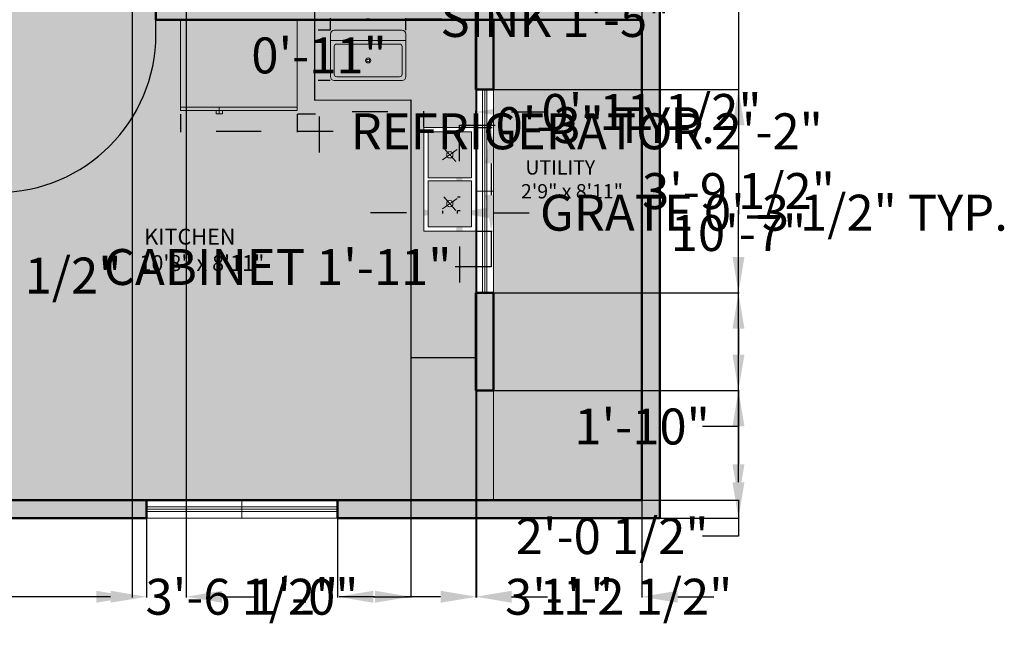
# Model space of a CAD drawing. Units: inches. Extents: x 339 to 824, y 73 to 445.
# Tile 3 of 5: x 605 to 824, y 73 to 213. Entities that reach past the tile are written whole.
import ezdxf

# ---------------------------------------------------------------- set-up
doc = ezdxf.new("R2010")
doc.units = ezdxf.units.IN
doc.header["$MEASUREMENT"] = 0
for name, color, linetype, lineweight in [('A-ANNO-DIMS', 2, 'Continuous', 18), ('A-AREA-IDEN', 7, 'Continuous', 25), ('A-DOOR', 3, 'Continuous', 25), ('A-EQPM', 9, 'Continuous', 20), ('A-EQPM-PATT', 96, 'Continuous', 13), ('A-FLOR-BNDY', 8, 'Continuous', 13), ('A-FLOR-CASE', 7, 'Continuous', 25), ('A-FLOR-FIXT', 9, 'Continuous', 20), ('A-FLOR-FIXT-PATT', 96, 'Continuous', 13), ('A-FLOR-PATT', 8, 'Continuous', 13), ('A-GLAZ', 4, 'Continuous', 18), ('A-WALL', 7, 'Continuous', 50), ('A-WALL-PATT', 1, 'Continuous', 13)]:
    doc.layers.add(name, color=color, linetype=linetype, lineweight=lineweight)
doc.layers.add('A-FLOR-CASE-PATT', color=18, linetype='Continuous', lineweight=13, true_color=0x000000)
doc.styles.get("Standard").update_dxf_attribs({"font": 'arial.ttf'})
doc.dimstyles.get("Standard").update_dxf_attribs({"dimtxt": 8, "dimasz": 8, "dimexe": 0.18, "dimexo": 0.0625, "dimgap": 0.09, "dimtad": 0, "dimtih": 1, "dimtoh": 1, "dimdec": 0, "dimzin": 0, "dimdsep": 46, "dimlunit": 3, "dimtxsty": 'Standard', "dimcen": 0.09, "dimadec": 0, "dimazin": 0, "dimtfac": 1, "dimtdec": 0, "dimtofl": 0, "dimtmove": 0, "dimatfit": 3, "dimfxl": 1, "dimtolj": 1, "dimtzin": 0, "dimarcsym": 0})

# ---------------------------------------------------------------- blocks, each defined once
blk = doc.blocks.new('*U3')
for p, q in [((0, 0), (0, 6)), ((40, 0), (40, 6))]:
    blk.add_line(p, q)
blk.add_lwpolyline([(0, 0), (0, -40), (1.75, -40), (1.75, 0)], close=True)
blk.add_arc((0, 0), 40, 270, 0)
blk = doc.blocks.new('Wall Cabinet - 18 x 36 in front')
for p, q in [((17.5, -1.5), (17.5, -16.5)), ((18.5, -16.5), (18.5, -1.5))]:
    blk.add_line(p, q)
blk.add_lwpolyline([(0, -18), (0, 0), (36, 0), (36, -18)], close=True)
for points in [[(17.5, -16.5), (1.5, -16.5), (1.5, -1.5), (17.5, -1.5)], [(18.5, -1.5), (34.5, -1.5), (34.5, -16.5), (18.5, -16.5)]]:
    blk.add_lwpolyline(points)
blk = doc.blocks.new('Sink-single - 30 in top')
blk.add_line((-15, -3.999996), (15, -3.999996))
for points in [[(-13.5, 0), (13.5, 0)], [(-15, -18.499996), (-15, -1.5)], [(15, -1.5), (15, -18.499996)], [(-13.5, -17.499996), (-13.5, -6.499996)], [(-12.5, -5.499996), (12.5, -5.499996)], [(13.5, -6.499996), (13.5, -17.499996)], [(12.5, -18.499996), (-12.5, -18.499996)], [(13.5, -19.999996), (-13.5, -19.999996)]]:
    blk.add_lwpolyline(points)
for radius in [1, 0.5]:
    blk.add_circle((0, -11.999996), radius)
for centre, radius, start, end in [((-13.5, -1.5), 1.5, 90, 180), ((13.5, -1.5), 1.5, 0, 90), ((-12.5, -6.499996), 1, 90, 180), ((12.5, -6.499996), 1, 0, 90), ((-13.5, -18.499996), 1.5, 180, 270), ((-12.5, -17.499996), 1, 180, 270), ((12.5, -17.499996), 1, 270, 0), ((13.5, -18.499996), 1.5, 270, 0)]:
    blk.add_arc(centre, radius, start, end)
blk = doc.blocks.new('Refrigerator-2 door - 36 in top')
for p, q in [((0, -26.999999), (36, -26.999999)), ((12, -26.999999), (12, -28.999999)), ((11, -27.999999), (11, -28.999999)), ((11, -28.999999), (13, -28.999999)), ((13, -28.999999), (13, -27.999999))]:
    blk.add_line(p, q)
blk.add_lwpolyline([(0, -27.999999), (0, 0), (36, 0), (36, -27.999999)], close=True)
blk = doc.blocks.new('COOKTOP-BURNER-GRATE')
for p, q in [((1.64, 1.15), (-1.64, -1.15)), ((0, 0), (-1.31, 1.51)), ((-1.31, 1.51), (1.31, -1.51)), ((0, 0), (1.64, 1.15))]:
    blk.add_line(p, q)
blk = doc.blocks.new('*D17')
at = {"layer": 'A-ANNO-DIMS', "color": 0, "lineweight": -2, "transparency": 16777216}
for p, q in [((561.97, 165.4), (561.97, 155.9)), ((578.48, 165.4), (578.48, 155.9)), ((569.97, 156.08), (570.48, 156.08)), ((578.48, 156.08), (586.48, 156.08))]:
    blk.add_line(p, q, dxfattribs=at)
at = {"layer": 'A-ANNO-DIMS', "color": 0, "transparency": 16777216}
for points in [[(569.97, 157.41), (569.97, 154.74), (561.97, 156.08)], [(570.48, 157.41), (570.48, 154.74), (578.48, 156.08)]]:
    blk.add_solid(points, dxfattribs=at)
at = {"layer": 'Defpoints', "color": 0, "transparency": 16777216}
for p in [(561.97, 165.46), (578.48, 165.46), (578.48, 156.08)]:
    blk.add_point(p, dxfattribs=at)
at = {"layer": 'A-ANNO-DIMS', "color": 0, "transparency": 16777216, "insert": (606.15, 156.08), "char_height": 8, "attachment_point": 5}
blk.add_mtext('\\A1;1\'-4 1/2"', dxfattribs=at)
blk = doc.blocks.new('*D22')
at = {"layer": 'A-ANNO-DIMS', "color": 0, "lineweight": -2, "transparency": 16777216}
for p, q in [((640.73, 192.04), (640.73, 188.02)), ((666.74, 192.04), (666.74, 188.02)), ((648.73, 188.2), (658.74, 188.2)), ((666.74, 188.2), (674.74, 188.2))]:
    blk.add_line(p, q, dxfattribs=at)
at = {"layer": 'A-ANNO-DIMS', "color": 0, "transparency": 16777216}
for points in [[(648.73, 189.54), (648.73, 186.87), (640.73, 188.2)], [(658.74, 189.54), (658.74, 186.87), (666.74, 188.2)]]:
    blk.add_solid(points, dxfattribs=at)
at = {"layer": 'Defpoints', "color": 0, "transparency": 16777216}
for p in [(640.73, 192.11), (666.74, 192.11), (666.74, 188.2)]:
    blk.add_point(p, dxfattribs=at)
at = {"layer": 'A-ANNO-DIMS', "color": 0, "transparency": 16777216, "insert": (731.21, 188.2), "char_height": 8, "attachment_point": 5}
blk.add_mtext('\\A1;REFRIGERATOR 2\'-2"', dxfattribs=at)
blk = doc.blocks.new('*D23')
at = {"layer": 'A-ANNO-DIMS', "color": 0, "lineweight": -2, "transparency": 16777216}
for p, q in [((670.64, 213.06), (670.64, 221.06)), ((670.64, 221.06), (678.64, 221.06)), ((666.81, 213.06), (670.82, 213.06)), ((670.64, 200.11), (670.64, 205.06)), ((666.81, 192.11), (670.82, 192.11))]:
    blk.add_line(p, q, dxfattribs=at)
at = {"layer": 'A-ANNO-DIMS', "color": 0, "transparency": 16777216}
for points in [[(669.31, 205.06), (671.98, 205.06), (670.64, 213.06)], [(669.31, 200.11), (671.98, 200.11), (670.64, 192.11)]]:
    blk.add_solid(points, dxfattribs=at)
at = {"layer": 'Defpoints', "color": 0, "transparency": 16777216}
for p in [(666.74, 213.06), (670.64, 213.06), (666.74, 192.11)]:
    blk.add_point(p, dxfattribs=at)
at = {"layer": 'A-ANNO-DIMS', "color": 0, "transparency": 16777216, "insert": (688.99, 221.06), "char_height": 8, "attachment_point": 5}
blk.add_mtext('\\A1;1\'-9"', dxfattribs=at)
blk = doc.blocks.new('*D24')
at = {"layer": 'A-ANNO-DIMS', "color": 0, "lineweight": -2, "transparency": 16777216}
for p, q in [((674.13, 210.76), (674.13, 213.4)), ((682.13, 213.22), (682.94, 213.22)), ((690.94, 210.76), (690.94, 213.4)), ((690.94, 213.22), (698.94, 213.22))]:
    blk.add_line(p, q, dxfattribs=at)
at = {"layer": 'A-ANNO-DIMS', "color": 0, "transparency": 16777216}
for points in [[(682.13, 214.56), (682.13, 211.89), (674.13, 213.22)], [(682.94, 214.56), (682.94, 211.89), (690.94, 213.22)]]:
    blk.add_solid(points, dxfattribs=at)
at = {"layer": 'Defpoints', "color": 0, "transparency": 16777216}
for p in [(690.94, 213.22), (674.13, 210.7), (690.94, 210.7)]:
    blk.add_point(p, dxfattribs=at)
at = {"layer": 'A-ANNO-DIMS', "color": 0, "transparency": 16777216, "insert": (724.24, 213.22), "char_height": 8, "attachment_point": 5}
blk.add_mtext('\\A1;SINK 1\'-5"', dxfattribs=at)
blk = doc.blocks.new('*D25')
at = {"layer": 'A-ANNO-DIMS', "color": 0, "lineweight": -2, "transparency": 16777216}
for p, q in [((671.61, 218.7), (671.61, 226.7)), ((674.07, 210.7), (671.43, 210.7)), ((674.07, 199.5), (671.43, 199.5)), ((671.61, 191.5), (671.61, 183.5))]:
    blk.add_line(p, q, dxfattribs=at)
at = {"layer": 'A-ANNO-DIMS', "color": 0, "transparency": 16777216}
for points in [[(670.28, 218.7), (672.95, 218.7), (671.61, 210.7)], [(670.28, 191.5), (672.95, 191.5), (671.61, 199.5)]]:
    blk.add_solid(points, dxfattribs=at)
at = {"layer": 'Defpoints', "color": 0, "transparency": 16777216}
for p in [(671.61, 210.7), (674.13, 210.7), (674.13, 199.5)]:
    blk.add_point(p, dxfattribs=at)
at = {"layer": 'A-ANNO-DIMS', "color": 0, "transparency": 16777216, "insert": (671.61, 205.1), "char_height": 8, "attachment_point": 5}
blk.add_mtext('\\A1;0\'-11"', dxfattribs=at)
blk = doc.blocks.new('*D26')
at = {"layer": 'A-ANNO-DIMS', "color": 0, "lineweight": -2, "transparency": 16777216}
for p, q in [((706.55, 189.05), (710.12, 189.05)), ((709.94, 181.05), (709.94, 173.99)), ((706.55, 165.99), (710.12, 165.99)), ((709.94, 165.99), (709.94, 157.99)), ((709.94, 157.99), (701.94, 157.99))]:
    blk.add_line(p, q, dxfattribs=at)
at = {"layer": 'A-ANNO-DIMS', "color": 0, "transparency": 16777216}
for points in [[(708.61, 181.05), (711.28, 181.05), (709.94, 189.05)], [(708.61, 173.99), (711.28, 173.99), (709.94, 165.99)]]:
    blk.add_solid(points, dxfattribs=at)
at = {"layer": 'Defpoints', "color": 0, "transparency": 16777216}
for p in [(706.48, 189.05), (706.48, 165.99), (709.94, 165.99)]:
    blk.add_point(p, dxfattribs=at)
at = {"layer": 'A-ANNO-DIMS', "color": 0, "transparency": 16777216, "insert": (662.39, 157.99), "char_height": 8, "attachment_point": 5}
blk.add_mtext('\\A1;CABINET 1\'-11"', dxfattribs=at)
blk = doc.blocks.new('*D27')
at = {"layer": 'A-ANNO-DIMS', "color": 0, "lineweight": -2, "transparency": 16777216}
for p, q in [((686.95, 192.51), (678.95, 192.51)), ((694.95, 189.11), (694.95, 192.69)), ((706.48, 189.11), (706.48, 192.69)), ((714.48, 192.51), (722.48, 192.51))]:
    blk.add_line(p, q, dxfattribs=at)
at = {"layer": 'A-ANNO-DIMS', "color": 0, "transparency": 16777216}
for points in [[(686.95, 193.84), (686.95, 191.18), (694.95, 192.51)], [(714.48, 193.84), (714.48, 191.18), (706.48, 192.51)]]:
    blk.add_solid(points, dxfattribs=at)
at = {"layer": 'Defpoints', "color": 0, "transparency": 16777216}
for p in [(706.48, 192.51), (694.95, 189.05), (706.48, 189.05)]:
    blk.add_point(p, dxfattribs=at)
at = {"layer": 'A-ANNO-DIMS', "color": 0, "transparency": 16777216, "insert": (745.64, 192.51), "char_height": 8, "attachment_point": 5}
blk.add_mtext('\\A1;0\'-11 1/2"', dxfattribs=at)
blk = doc.blocks.new('*D28')
at = {"layer": 'A-ANNO-DIMS', "color": 0, "lineweight": -2, "transparency": 16777216}
for p, q in [((691.08, 170.08), (683.08, 170.08)), ((699.08, 170.51), (699.08, 169.9)), ((702.35, 170.51), (702.35, 169.9)), ((710.35, 170.08), (718.35, 170.08))]:
    blk.add_line(p, q, dxfattribs=at)
at = {"layer": 'A-ANNO-DIMS', "color": 0, "transparency": 16777216}
for points in [[(691.08, 171.41), (691.08, 168.74), (699.08, 170.08)], [(710.35, 171.41), (710.35, 168.74), (702.35, 170.08)]]:
    blk.add_solid(points, dxfattribs=at)
at = {"layer": 'Defpoints', "color": 0, "transparency": 16777216}
for p in [(699.08, 170.57), (702.35, 170.57), (702.35, 170.08)]:
    blk.add_point(p, dxfattribs=at)
at = {"layer": 'A-ANNO-DIMS', "color": 0, "transparency": 16777216, "insert": (772.88, 170.08), "char_height": 8, "attachment_point": 5}
blk.add_mtext('\\A1;GRATE 0\'-3 1/2" TYP.', dxfattribs=at)
blk = doc.blocks.new('*D29')
at = {"layer": 'A-ANNO-DIMS', "color": 0, "lineweight": -2, "transparency": 16777216}
for p, q in [((702.84, 181.58), (702.84, 189.58)), ((702.84, 189.58), (710.84, 189.58)), ((702.42, 173.58), (703.02, 173.58)), ((702.42, 170.57), (703.02, 170.57)), ((702.84, 162.57), (702.84, 154.57))]:
    blk.add_line(p, q, dxfattribs=at)
at = {"layer": 'A-ANNO-DIMS', "color": 0, "transparency": 16777216}
for points in [[(701.51, 181.58), (704.18, 181.58), (702.84, 173.58)], [(701.51, 162.57), (704.18, 162.57), (702.84, 170.57)]]:
    blk.add_solid(points, dxfattribs=at)
at = {"layer": 'Defpoints', "color": 0, "transparency": 16777216}
for p in [(702.35, 173.58), (702.84, 173.58), (702.35, 170.57)]:
    blk.add_point(p, dxfattribs=at)
at = {"layer": 'A-ANNO-DIMS', "color": 0, "transparency": 16777216, "insert": (735.32, 189.58), "char_height": 8, "attachment_point": 5}
blk.add_mtext('\\A1;0\'-3" TYP.', dxfattribs=at)
blk = doc.blocks.new('*D32')
at = {"layer": 'A-ANNO-DIMS', "color": 0, "lineweight": -2, "transparency": 16777216}
for p, q in [((546.07, 102), (546.07, 84.38)), ((633.18, 102), (633.18, 84.38)), ((554.07, 84.56), (578.93, 84.56)), ((625.18, 84.56), (600.31, 84.56))]:
    blk.add_line(p, q, dxfattribs=at)
at = {"layer": 'A-ANNO-DIMS', "color": 0, "transparency": 16777216}
for points in [[(554.07, 85.89), (554.07, 83.23), (546.07, 84.56)], [(625.18, 85.89), (625.18, 83.23), (633.18, 84.56)]]:
    blk.add_solid(points, dxfattribs=at)
at = {"layer": 'Defpoints', "color": 0, "transparency": 16777216}
for p in [(546.07, 102.06), (633.18, 102.06), (633.18, 84.56)]:
    blk.add_point(p, dxfattribs=at)
at = {"layer": 'A-ANNO-DIMS', "color": 0, "transparency": 16777216, "insert": (589.62, 84.56), "char_height": 8, "attachment_point": 5}
blk.add_mtext('\\A1;7\'-3"', dxfattribs=at)
blk = doc.blocks.new('*D33')
at = {"layer": 'A-ANNO-DIMS', "color": 0, "lineweight": -2, "transparency": 16777216}
for p, q in [((633.18, 102), (633.18, 84.38)), ((675.71, 102), (675.71, 84.38)), ((625.18, 84.56), (617.18, 84.56)), ((683.71, 84.56), (691.71, 84.56))]:
    blk.add_line(p, q, dxfattribs=at)
at = {"layer": 'A-ANNO-DIMS', "color": 0, "transparency": 16777216}
for points in [[(625.18, 85.89), (625.18, 83.23), (633.18, 84.56)], [(683.71, 85.89), (683.71, 83.23), (675.71, 84.56)]]:
    blk.add_solid(points, dxfattribs=at)
at = {"layer": 'Defpoints', "color": 0, "transparency": 16777216}
for p in [(633.18, 102.06), (675.71, 102.06), (675.71, 84.56)]:
    blk.add_point(p, dxfattribs=at)
at = {"layer": 'A-ANNO-DIMS', "color": 0, "transparency": 16777216, "insert": (654.44, 84.56), "char_height": 8, "attachment_point": 5}
blk.add_mtext('\\A1;3\'-6 1/2"', dxfattribs=at)
blk = doc.blocks.new('*D36')
at = {"layer": 'A-ANNO-DIMS', "color": 0, "lineweight": -2, "transparency": 16777216}
for p, q in [((747.55, 229.04), (765.16, 229.04)), ((764.98, 221.04), (764.98, 169.72)), ((764.98, 110.06), (764.98, 161.37)), ((747.55, 102.06), (765.16, 102.06))]:
    blk.add_line(p, q, dxfattribs=at)
at = {"layer": 'A-ANNO-DIMS', "color": 0, "transparency": 16777216}
for points in [[(763.65, 221.04), (766.32, 221.04), (764.98, 229.04)], [(763.65, 110.06), (766.32, 110.06), (764.98, 102.06)]]:
    blk.add_solid(points, dxfattribs=at)
at = {"layer": 'Defpoints', "color": 0, "transparency": 16777216}
for p in [(747.48, 229.04), (764.98, 229.04), (747.48, 102.06)]:
    blk.add_point(p, dxfattribs=at)
at = {"layer": 'A-ANNO-DIMS', "color": 0, "transparency": 16777216, "insert": (764.98, 165.55), "char_height": 8, "attachment_point": 5}
blk.add_mtext('\\A1;10\'-7"', dxfattribs=at)
blk = doc.blocks.new('*D39')
at = {"layer": 'A-ANNO-DIMS', "color": 0, "lineweight": -2, "transparency": 16777216}
for p, q in [((706.66, 342), (706.66, 84.38)), ((743.48, 342), (743.48, 84.38)), ((698.66, 84.56), (690.66, 84.56)), ((751.48, 84.56), (759.48, 84.56))]:
    blk.add_line(p, q, dxfattribs=at)
at = {"layer": 'A-ANNO-DIMS', "color": 0, "transparency": 16777216}
for points in [[(698.66, 85.89), (698.66, 83.23), (706.66, 84.56)], [(751.48, 85.89), (751.48, 83.23), (743.48, 84.56)]]:
    blk.add_solid(points, dxfattribs=at)
at = {"layer": 'Defpoints', "color": 0, "transparency": 16777216}
for p in [(706.66, 342.06), (743.48, 342.06), (743.48, 84.56)]:
    blk.add_point(p, dxfattribs=at)
at = {"layer": 'A-ANNO-DIMS', "color": 0, "transparency": 16777216, "insert": (725.07, 84.56), "char_height": 8, "attachment_point": 5}
blk.add_mtext('\\A1;3\'-1"', dxfattribs=at)
blk = doc.blocks.new('*D53')
at = {"layer": 'A-ANNO-DIMS', "color": 0, "lineweight": -2, "transparency": 16777216}
for p, q in [((630, 375), (630, 84.38)), ((642, 375), (642, 84.38)), ((622, 84.56), (614, 84.56)), ((650, 84.56), (658, 84.56))]:
    blk.add_line(p, q, dxfattribs=at)
at = {"layer": 'A-ANNO-DIMS', "color": 0, "transparency": 16777216}
for points in [[(622, 85.89), (622, 83.23), (630, 84.56)], [(650, 85.89), (650, 83.23), (642, 84.56)]]:
    blk.add_solid(points, dxfattribs=at)
at = {"layer": 'Defpoints', "color": 0, "transparency": 16777216}
for p in [(630, 375.06), (642, 375.06), (642, 84.56)]:
    blk.add_point(p, dxfattribs=at)
at = {"layer": 'A-ANNO-DIMS', "color": 0, "transparency": 16777216, "insert": (668.35, 84.56), "char_height": 8, "attachment_point": 5}
blk.add_mtext('\\A1;1\'-0"', dxfattribs=at)
blk = doc.blocks.new('*D56')
at = {"layer": 'A-ANNO-DIMS', "color": 0, "lineweight": -2, "transparency": 16777216}
for p, q in [((710.55, 130.47), (765.16, 130.47)), ((764.98, 122.47), (764.98, 114.06)), ((710.55, 106.06), (765.16, 106.06)), ((764.98, 106.06), (764.98, 98.06)), ((764.98, 98.06), (756.98, 98.06))]:
    blk.add_line(p, q, dxfattribs=at)
at = {"layer": 'A-ANNO-DIMS', "color": 0, "transparency": 16777216}
for points in [[(763.65, 122.47), (766.32, 122.47), (764.98, 130.47)], [(763.65, 114.06), (766.32, 114.06), (764.98, 106.06)]]:
    blk.add_solid(points, dxfattribs=at)
at = {"layer": 'Defpoints', "color": 0, "transparency": 16777216}
for p in [(710.48, 130.47), (710.48, 106.06), (764.98, 106.06)]:
    blk.add_point(p, dxfattribs=at)
at = {"layer": 'A-ANNO-DIMS', "color": 0, "transparency": 16777216, "insert": (736.87, 98.06), "char_height": 8, "attachment_point": 5}
blk.add_mtext('\\A1;2\'-0 1/2"', dxfattribs=at)
blk = doc.blocks.new('*D64')
at = {"layer": 'A-ANNO-DIMS', "color": 0, "lineweight": -2, "transparency": 16777216}
for p, q in [((710.55, 197.55), (765.16, 197.55)), ((764.98, 189.55), (764.98, 179.13)), ((764.98, 160.25), (764.98, 170.67)), ((710.55, 152.25), (765.16, 152.25))]:
    blk.add_line(p, q, dxfattribs=at)
at = {"layer": 'A-ANNO-DIMS', "color": 0, "transparency": 16777216}
for points in [[(763.65, 189.55), (766.32, 189.55), (764.98, 197.55)], [(763.65, 160.25), (766.32, 160.25), (764.98, 152.25)]]:
    blk.add_solid(points, dxfattribs=at)
at = {"layer": 'Defpoints', "color": 0, "transparency": 16777216}
for p in [(710.48, 197.55), (710.48, 152.25), (764.98, 152.25)]:
    blk.add_point(p, dxfattribs=at)
at = {"layer": 'A-ANNO-DIMS', "color": 0, "transparency": 16777216, "insert": (764.98, 174.9), "char_height": 8, "attachment_point": 5}
blk.add_mtext('\\A1;3\'-9 1/2"', dxfattribs=at)
blk = doc.blocks.new('*D65')
at = {"layer": 'A-ANNO-DIMS', "color": 0, "lineweight": -2, "transparency": 16777216}
for p, q in [((710.55, 152.25), (765.16, 152.25)), ((764.98, 144.25), (764.98, 138.47)), ((710.55, 130.47), (765.16, 130.47)), ((764.98, 130.47), (764.98, 122.47)), ((764.98, 122.47), (756.98, 122.47))]:
    blk.add_line(p, q, dxfattribs=at)
at = {"layer": 'A-ANNO-DIMS', "color": 0, "transparency": 16777216}
for points in [[(763.65, 144.25), (766.32, 144.25), (764.98, 152.25)], [(763.65, 138.47), (766.32, 138.47), (764.98, 130.47)]]:
    blk.add_solid(points, dxfattribs=at)
at = {"layer": 'Defpoints', "color": 0, "transparency": 16777216}
for p in [(710.48, 152.25), (710.48, 130.47), (764.98, 130.47)]:
    blk.add_point(p, dxfattribs=at)
at = {"layer": 'A-ANNO-DIMS', "color": 0, "transparency": 16777216, "insert": (743.53, 122.47), "char_height": 8, "attachment_point": 5}
blk.add_mtext('\\A1;1\'-10"', dxfattribs=at)
blk = doc.blocks.new('*D66')
at = {"layer": 'A-ANNO-DIMS', "color": 0, "lineweight": -2, "transparency": 16777216}
for p, q in [((692.06, 137.73), (692.06, 84.38)), ((706.48, 137.73), (706.48, 84.38)), ((684.06, 84.56), (676.06, 84.56)), ((714.48, 84.56), (722.48, 84.56))]:
    blk.add_line(p, q, dxfattribs=at)
at = {"layer": 'A-ANNO-DIMS', "color": 0, "transparency": 16777216}
for points in [[(684.06, 85.89), (684.06, 83.23), (692.06, 84.56)], [(714.48, 85.89), (714.48, 83.23), (706.48, 84.56)]]:
    blk.add_solid(points, dxfattribs=at)
at = {"layer": 'Defpoints', "color": 0, "transparency": 16777216}
for p in [(692.06, 137.8), (706.48, 137.8), (706.48, 84.56)]:
    blk.add_point(p, dxfattribs=at)
at = {"layer": 'A-ANNO-DIMS', "color": 0, "transparency": 16777216, "insert": (742.15, 84.56), "char_height": 8, "attachment_point": 5}
blk.add_mtext('\\A1;1\'-2 1/2"', dxfattribs=at)

msp = doc.modelspace()

# ---------------------------------------------------------------- hatches: boundary and pattern name
at = {"layer": 'A-EQPM-PATT'}
h = msp.add_hatch(color=256, dxfattribs=at)
h.dxf.hatch_style = 1
h.paths.add_polyline_path([(666.74, 213.06), (640.73, 213.06), (640.73, 193.55), (666.74, 193.55)])
h = msp.add_hatch(color=256, dxfattribs=at)
h.dxf.hatch_style = 1
h.paths.add_polyline_path([(705.52, 177.84), (705.52, 188.09), (695.91, 188.09), (695.91, 177.84)])
h.paths.add_polyline_path([(700.02, 182.97, -1), (701.42, 182.97, -1)], flags=16)
h = msp.add_hatch(color=256, dxfattribs=at)
h.dxf.hatch_style = 1
h.paths.add_polyline_path([(695.91, 177.2), (695.91, 166.95), (705.52, 166.95), (705.52, 177.2)])
h.paths.add_polyline_path([(701.42, 172.07, -1), (700.02, 172.07, -1)], flags=16)
at = {"layer": 'A-FLOR-CASE-PATT'}
h = msp.add_hatch(color=256, dxfattribs=at)
h.dxf.hatch_style = 1
h.paths.add_polyline_path([(706.48, 213.06), (670.62, 213.06), (670.62, 195.11), (692.06, 195.19), (692.06, 137.8), (706.48, 137.8), (706.48, 152.25), (706.48, 165.99), (694.95, 165.99), (694.95, 189.05), (706.48, 189.05), (706.48, 202.79)])
h.paths.add_polyline_path([(690.94, 200.34, -0.414214), (690.1, 199.5), (674.97, 199.5, -0.414214), (674.13, 200.34), (674.13, 209.86, -0.414214), (674.97, 210.7), (690.1, 210.7, -0.414214), (690.94, 209.86)], flags=16)
h.paths.add_polyline_path([(690.1, 200.9, -0.414214), (689.54, 200.34), (675.53, 200.34, -0.414214), (674.97, 200.9), (674.97, 207.06, -0.414214), (675.53, 207.62), (689.54, 207.62, -0.414214), (690.1, 207.06)], flags=0)
h.paths.add_polyline_path([(682.26, 203.98, -1), (682.82, 203.98, -1)], flags=0)
h.paths.add_polyline_path([(681.98, 203.98, -1), (683.1, 203.98, -1)], flags=0)
at = {"layer": 'A-FLOR-FIXT-PATT'}
h = msp.add_hatch(color=256, dxfattribs=at)
h.dxf.hatch_style = 1
h.paths.add_polyline_path([(674.97, 210.7, 0.414214), (674.13, 209.86), (674.13, 208.46), (690.94, 208.46), (690.94, 209.86, 0.414214), (690.1, 210.7)])
h = msp.add_hatch(color=256, dxfattribs=at)
h.dxf.hatch_style = 1
h.paths.add_polyline_path([(690.1, 207.06, 0.414214), (689.54, 207.62), (675.53, 207.62, 0.414214), (674.97, 207.06), (674.97, 200.9, 0.414214), (675.53, 200.34), (689.54, 200.34, 0.414214), (690.1, 200.9)], flags=16)
h.paths.add_polyline_path([(690.94, 208.46), (674.13, 208.46), (674.13, 200.34, 0.414214), (674.97, 199.5), (690.1, 199.5, 0.414214), (690.94, 200.34)])
h.paths.add_polyline_path([(682.26, 203.98, -1), (682.82, 203.98, -1)], flags=0)
h = msp.add_hatch(color=256, dxfattribs=at)
h.dxf.hatch_style = 1
h.paths.add_polyline_path([(681.98, 203.98, 1), (683.1, 203.98, 1)], flags=16)
h.paths.add_polyline_path([(682.26, 203.98, -1), (682.82, 203.98, -1)], flags=0)
h.paths.add_polyline_path([(689.54, 200.34, 0.414214), (690.1, 200.9), (690.1, 207.06, 0.414214), (689.54, 207.62), (675.53, 207.62, 0.414214), (674.97, 207.06), (674.97, 200.9, 0.414214), (675.53, 200.34)])
at = {"layer": 'A-FLOR-PATT'}
h = msp.add_hatch(color=256, dxfattribs=at)
h.dxf.hatch_style = 1
h.paths.add_polyline_path([(578.48, 106.06), (710.48, 106.06), (710.48, 130.47), (706.48, 130.47), (706.48, 137.8), (692.06, 137.8), (692.06, 195.19), (670.62, 195.11), (670.62, 213.06), (635.29, 213.06), (635.29, 217.06), (600.11, 217.06), (600.11, 213.06), (582.48, 213.06), (582.48, 147.67), (578.48, 147.67)])
h.paths.add_polyline_path([(600.11, 174.62), (600.11, 209.78), (601.65, 209.78), (601.65, 174.62)], flags=16)
h.paths.add_polyline_path([(630.19, 155.1), (658.99, 155.1), (658.99, 168.27), (630.19, 168.27)], flags=24)
h = msp.add_hatch(color=256, dxfattribs=at)
h.dxf.hatch_style = 1
h.paths.add_polyline_path([(710.48, 106.06), (710.48, 130.47), (706.48, 130.47), (706.48, 137.8), (692.06, 137.8), (692.06, 195.19), (670.62, 195.11), (670.62, 213.06), (635.29, 213.06), (635.29, 217.06), (600.11, 217.06), (600.11, 213.06), (582.48, 213.06), (582.48, 147.67), (582.91, 106.06)])
h.paths.add_polyline_path([(601.65, 174.62), (600.11, 174.62), (600.11, 209.78), (601.65, 209.78)], flags=16)
h.paths.add_polyline_path([(630.19, 155.1), (658.99, 155.1), (658.99, 168.27), (630.19, 168.27)], flags=24)
h = msp.add_hatch(color=256, dxfattribs=at)
h.dxf.hatch_style = 1
h.paths.add_polyline_path([(743.48, 213.06), (710.48, 213.06), (710.48, 197.55), (710.48, 152.25), (710.48, 106.06), (743.48, 106.06)])
h.paths.add_polyline_path([(715.64, 171.51), (739.16, 171.51), (739.16, 183.4), (715.64, 183.4)], flags=24)
h = msp.add_hatch(color=256, dxfattribs=at)
h.dxf.hatch_style = 1
h.paths.add_polyline_path([(710.48, 213.06), (710.48, 197.55), (710.48, 152.25), (710.48, 106.06), (743.48, 106.06), (743.48, 213.06)])
h.paths.add_polyline_path([(715.64, 171.51), (739.16, 171.51), (739.16, 183.4), (715.64, 183.4)], flags=24)
at = {"layer": 'A-WALL-PATT'}
h = msp.add_hatch(color=256, dxfattribs=at)
h.dxf.hatch_style = 1
h.paths.add_polyline_path([(675.71, 106.06), (675.71, 102.06), (743.48, 102.06), (747.48, 102.06), (747.48, 229.04), (743.48, 229.04), (743.48, 217.06), (660.4, 217.06), (635.29, 217.06), (635.29, 213.06), (743.48, 213.06), (743.48, 106.06)])
h = msp.add_hatch(color=256, dxfattribs=at)
h.dxf.hatch_style = 1
h.paths.add_polyline_path([(710.48, 213.06), (706.48, 213.06), (706.48, 197.55), (710.48, 197.55), (710.48, 202.79)])
h = msp.add_hatch(color=256, dxfattribs=at)
h.dxf.hatch_style = 1
h.paths.add_polyline_path([(706.48, 130.47), (710.48, 130.47), (710.48, 152.25), (706.48, 152.25)])
h = msp.add_hatch(color=256, dxfattribs=at)
h.dxf.hatch_style = 1
h.paths.add_polyline_path([(546.07, 106.06), (546.07, 102.06), (633.18, 102.06), (633.18, 106.06), (625.18, 106.06)])

# ---------------------------------------------------------------- linework, layer by layer
at = {"layer": 'A-EQPM'}
for centre in [(700.72, 182.97), (700.72, 172.07), (700.72, 172.07)]:
    msp.add_circle(centre, 0.697, dxfattribs=at)
at = {"layer": 'A-FLOR-BNDY'}
msp.add_line((710.48, 174.9), (710.48, 106.06), dxfattribs=at)
at = {"layer": 'A-FLOR-CASE'}
for p, q in [((670.62, 213.06), (670.62, 195.11)), ((670.62, 195.11), (692.06, 195.19)), ((692.06, 195.19), (692.06, 137.8)), ((692.06, 137.8), (706.48, 137.8))]:
    msp.add_line(p, q, dxfattribs=at)
at = {"layer": 'A-GLAZ'}
for p, q in [((706.48, 202.79), (706.48, 152.25)), ((710.48, 202.79), (710.48, 152.25)), ((707.98, 197.55), (707.98, 152.25)), ((708.48, 197.55), (708.48, 152.25)), ((708.98, 197.55), (708.98, 152.25)), ((706.48, 174.9), (710.48, 174.9)), ((710.48, 152.25), (706.48, 152.25)), ((654.44, 106.06), (654.44, 102.06)), ((675.71, 106.06), (675.71, 102.06)), ((633.18, 104.56), (675.71, 104.56)), ((633.18, 104.06), (675.71, 104.06)), ((633.18, 103.56), (675.71, 103.56)), ((625.18, 102.06), (675.71, 102.06))]:
    msp.add_line(p, q, dxfattribs=at)
at = {"layer": 'A-WALL'}
for p, q in [((747.48, 229.04), (747.48, 102.06)), ((635.29, 213.06), (635.29, 217.06)), ((635.29, 213.06), (743.48, 213.06)), ((706.48, 197.55), (706.48, 213.06)), ((710.48, 197.55), (710.48, 213.06)), ((743.48, 106.06), (743.48, 213.06)), ((706.48, 197.55), (710.48, 197.55)), ((706.48, 130.47), (706.48, 152.25)), ((706.48, 152.25), (710.48, 152.25)), ((710.48, 130.47), (710.48, 152.25)), ((710.48, 130.47), (706.48, 130.47)), ((532.64, 106.06), (633.18, 106.06)), ((578.48, 106.06), (743.48, 106.06)), ((633.18, 106.06), (633.18, 102.06)), ((675.71, 106.06), (675.71, 102.06)), ((675.71, 106.06), (743.48, 106.06)), ((546.07, 102.06), (633.18, 102.06)), ((675.71, 102.06), (743.48, 102.06)), ((747.48, 102.06), (743.48, 102.06))]:
    msp.add_line(p, q, dxfattribs=at)

# ---------------------------------------------------------------- block references
at = {"layer": 'A-DOOR', "xscale": 0.8792070118950395, "yscale": 0.8792070118950395, "zscale": 0.8792070118950395}
msp.add_blockref('*U3', (600.11, 209.78), dxfattribs=at)
at = {"layer": 'A-EQPM', "xscale": 0.7225888694948884, "yscale": 0.7225888694948884, "zscale": 0.7225888694948884}
msp.add_blockref('Refrigerator-2 door - 36 in top', (640.73, 213.06), dxfattribs=at)
at = {"layer": 'A-EQPM', "xscale": 0.6406482971506487, "yscale": 0.6406482971506487, "zscale": 0.6406482971506487, "rotation": 270}
msp.add_blockref('Wall Cabinet - 18 x 36 in front', (706.48, 189.05), dxfattribs=at)
at = {"layer": 'A-EQPM'}
for p in [(700.72, 182.97), (700.72, 172.07)]:
    msp.add_blockref('COOKTOP-BURNER-GRATE', p, dxfattribs=at)
at = {"layer": 'A-FLOR-FIXT', "xscale": 0.5601866757973277, "yscale": 0.5601866757973277, "zscale": 0.5601866757973277}
msp.add_blockref('Sink-single - 30 in top', (682.54, 210.7), dxfattribs=at)

# ---------------------------------------------------------------- texts
at = {"layer": 'A-AREA-IDEN', "attachment_point": 1}
for s, width, gutter_width, insert, char_height in [(' UTILITY\\P2\'9" x 8\'11"', 35.4655, 15.92, (716.57, 181.76), 3.1844), (' KITCHEN\\P10\'8" x 8\'11"', 39.2974, 17.64, (631.61, 166.51), 3.5285)]:
    msp.add_mtext_dynamic_manual_height_columns(s, width=width, gutter_width=gutter_width, heights=[0], dxfattribs=dict(at, insert=insert, char_height=char_height))

# ---------------------------------------------------------------- dimensions: what is measured, and where the dimension line sits
at = {"layer": 'A-ANNO-DIMS'}
for base, p1, p2, picture, middle in [((642, 84.56), (630, 375.06), (642, 375.06), '*D53', (668.35, 84.56)), ((743.48, 84.56), (706.66, 342.06), (743.48, 342.06), '*D39', (725.07, 84.56)), ((706.48, 192.51), (694.95, 189.05), (706.48, 189.05), '*D27', (745.64, 192.51)), ((578.48, 156.08), (561.97, 165.46), (578.48, 165.46), '*D17', (606.15, 156.08)), ((706.48, 84.56), (692.06, 137.8), (706.48, 137.8), '*D66', (742.15, 84.56)), ((633.18, 84.56), (546.07, 102.06), (633.18, 102.06), '*D32', (589.62, 84.56)), ((675.71, 84.56), (633.18, 102.06), (675.71, 102.06), '*D33', (654.44, 84.56))]:
    dim = msp.add_linear_dim(base=base, p1=p1, p2=p2, dimstyle='Standard', override={"dimdec": 1, "dimlfac": 1, "dimrnd": 0, "dimzin": 1, "dimdsep": 46, "dimlunit": 4, "dimfrac": 2}, dxfattribs=at)
    dim.commit()
    dim.dimension.update_dxf_attribs({"geometry": picture, "text_midpoint": middle})
for base, p1, p2, picture, middle in [((764.98, 229.04), (747.48, 102.06), (747.48, 229.04), '*D36', (764.98, 165.55)), ((671.61, 210.7), (674.13, 199.5), (674.13, 210.7), '*D25', (671.61, 205.1)), ((670.6446, 213.0602), (666.7427, 192.1052), (666.7427, 213.0602), '*D23', (688.9911, 221.0602)), ((764.98, 152.25), (710.48, 197.55), (710.48, 152.25), '*D64', (764.98, 174.9)), ((764.98, 130.47), (710.48, 152.25), (710.48, 130.47), '*D65', (743.53, 122.47)), ((764.98, 106.06), (710.48, 130.47), (710.48, 106.06), '*D56', (736.87, 98.06))]:
    dim = msp.add_linear_dim(base=base, p1=p1, p2=p2, angle=90, dimstyle='Standard', override={"dimdec": 1, "dimlfac": 1, "dimrnd": 0, "dimzin": 1, "dimdsep": 46, "dimlunit": 4, "dimfrac": 2}, dxfattribs=at)
    dim.commit()
    dim.dimension.update_dxf_attribs({"geometry": picture, "text_midpoint": middle})
for base, p1, p2, text, picture, middle in [((690.94, 213.22), (674.13, 210.7), (690.94, 210.7), 'SINK <>', '*D24', (724.24, 213.22)), ((666.74, 188.2), (640.73, 192.11), (666.74, 192.11), 'REFRIGERATOR <>', '*D22', (731.21, 188.2)), ((702.35, 170.08), (699.08, 170.57), (702.35, 170.57), 'GRATE <> TYP.', '*D28', (772.88, 170.08))]:
    dim = msp.add_linear_dim(base=base, p1=p1, p2=p2, text=text, dimstyle='Standard', override={"dimdec": 1, "dimlfac": 1, "dimrnd": 0, "dimzin": 1, "dimdsep": 46, "dimlunit": 4, "dimfrac": 2}, dxfattribs=at)
    dim.commit()
    dim.dimension.update_dxf_attribs({"geometry": picture, "text_midpoint": middle})
for base, p1, p2, angle, text, picture, middle in [((702.84, 173.58), (702.35, 170.57), (702.35, 173.58), 90, '<> TYP.', '*D29', (735.32, 189.58)), ((709.94, 165.99), (706.48, 189.05), (706.48, 165.99), 270, 'CABINET <>', '*D26', (662.39, 157.99))]:
    dim = msp.add_linear_dim(base=base, p1=p1, p2=p2, angle=angle, text=text, dimstyle='Standard', override={"dimdec": 1, "dimlfac": 1, "dimrnd": 0, "dimzin": 1, "dimdsep": 46, "dimlunit": 4, "dimfrac": 2}, dxfattribs=at)
    dim.commit()
    dim.dimension.update_dxf_attribs({"geometry": picture, "text_midpoint": middle})

doc.saveas('drawing.dxf')
